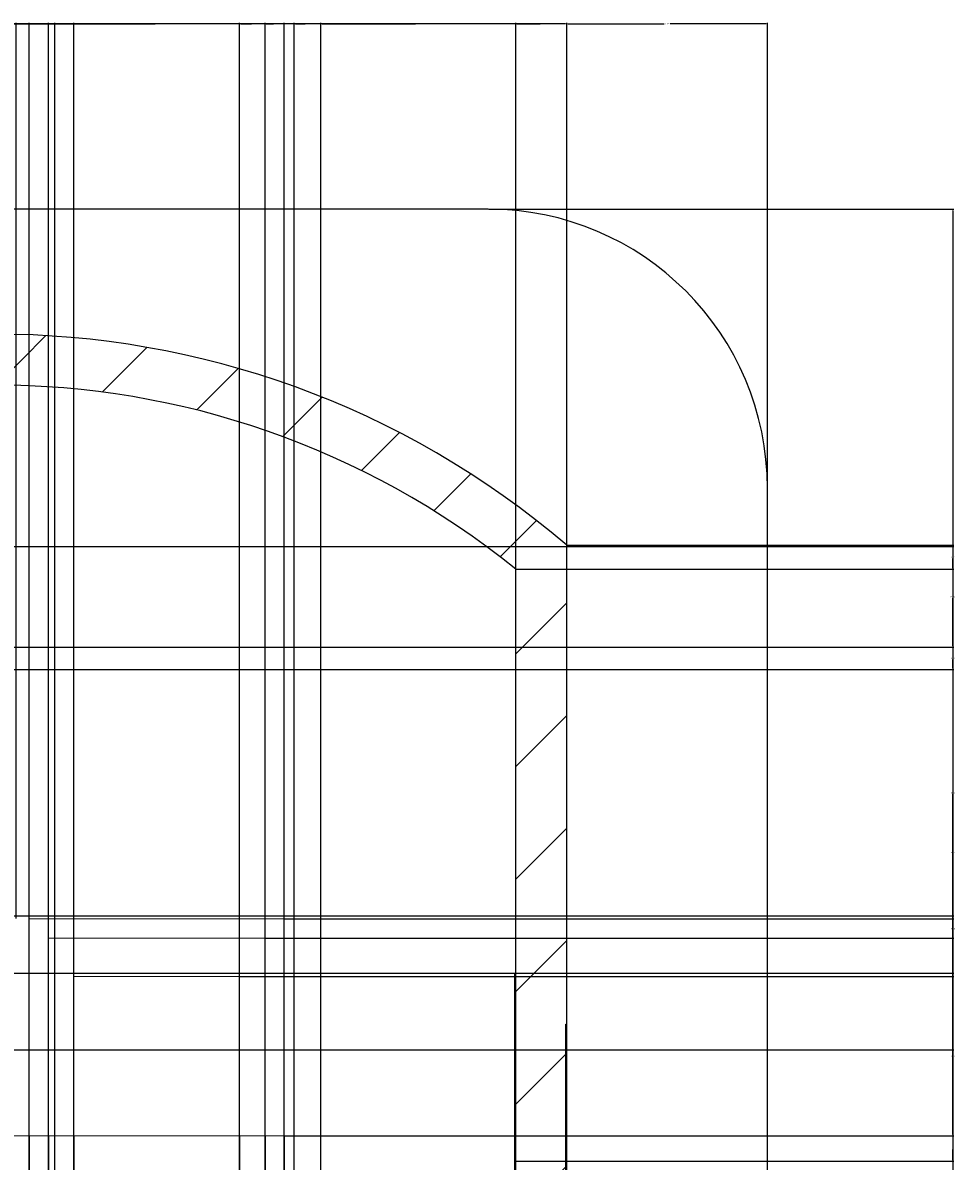
# Model space of a CAD drawing. Units: inches. Extents: x -14 to 375, y -86 to 549.
# Tile 12 of 12: x 228 to 375, y 336 to 515. Entities that reach past the tile are written whole.
import ezdxf

# ---------------------------------------------------------------- set-up
doc = ezdxf.new("R2010")
doc.units = ezdxf.units.IN
doc.header["$MEASUREMENT"] = 0
for name, color, linetype, lineweight in [('A-ANNO-DIMS', 2, 'Continuous', 18), ('A-DOOR', 3, 'Continuous', 18), ('A-ELEV', 7, 'Continuous', 25), ('A-ELEV-PATT', 8, 'Continuous', 13), ('A-ELEV-RAIL', 8, 'Continuous', 18)]:
    doc.layers.add(name, color=color, linetype=linetype, lineweight=lineweight)
doc.styles.get("Standard").update_dxf_attribs({"font": 'arial.ttf'})
doc.dimstyles.get("Standard").update_dxf_attribs({"dimtxt": 0.18, "dimasz": 0.18, "dimexe": 0.18, "dimexo": 0.0625, "dimgap": 0.09, "dimtad": 0, "dimtih": 1, "dimtoh": 1, "dimdec": 4, "dimzin": 0, "dimdsep": 46, "dimtxsty": 'Standard', "dimcen": 0.09, "dimadec": 0, "dimazin": 0, "dimtfac": 1, "dimtdec": 4, "dimtofl": 0, "dimtmove": 0, "dimatfit": 3, "dimfxl": 1, "dimtolj": 1, "dimtzin": 0, "dimarcsym": 0})

# ---------------------------------------------------------------- blocks, each defined once
blk = doc.blocks.new('*D8')
at = {"layer": 'A-ANNO-DIMS', "color": 0, "lineweight": -2, "transparency": 16777216}
for p, q in [((134.23, 433.23), (134.23, 515.24)), ((134.41, 515.06), (223.55, 515.06)), ((313.59, 515.06), (224.46, 515.06)), ((313.77, 433.23), (313.77, 515.24))]:
    blk.add_line(p, q, dxfattribs=at)
at = {"layer": 'A-ANNO-DIMS', "color": 0, "transparency": 16777216}
for points in [[(134.41, 515.09), (134.41, 515.03), (134.23, 515.06)], [(313.59, 515.09), (313.59, 515.03), (313.77, 515.06)]]:
    blk.add_solid(points, dxfattribs=at)
at = {"layer": 'Defpoints', "color": 0, "transparency": 16777216}
for p in [(313.77, 515.06), (134.23, 433.17), (313.77, 433.17)]:
    blk.add_point(p, dxfattribs=at)
at = {"layer": 'A-ANNO-DIMS', "color": 0, "transparency": 16777216, "insert": (224, 515.06), "char_height": 0.18, "attachment_point": 5}
blk.add_mtext('\\A1;179.54', dxfattribs=at)
blk = doc.blocks.new('*D9')
at = {"layer": 'A-ANNO-DIMS', "color": 0, "lineweight": -2, "transparency": 16777216}
for p, q in [((313.77, 433.23), (313.77, 515.24)), ((313.95, 515.06), (329.05, 515.06)), ((345.08, 515.06), (329.98, 515.06)), ((345.26, 442.21), (345.26, 515.24))]:
    blk.add_line(p, q, dxfattribs=at)
at = {"layer": 'A-ANNO-DIMS', "color": 0, "transparency": 16777216}
for points in [[(313.95, 515.09), (313.95, 515.03), (313.77, 515.06)], [(345.08, 515.09), (345.08, 515.03), (345.26, 515.06)]]:
    blk.add_solid(points, dxfattribs=at)
at = {"layer": 'Defpoints', "color": 0, "transparency": 16777216}
for p in [(345.26, 515.06), (345.26, 442.15), (313.77, 433.17)]:
    blk.add_point(p, dxfattribs=at)
at = {"layer": 'A-ANNO-DIMS', "color": 0, "transparency": 16777216, "insert": (329.52, 515.06), "char_height": 0.18, "attachment_point": 5}
blk.add_mtext('\\A1;31.495', dxfattribs=at)
blk = doc.blocks.new('*D10')
at = {"layer": 'A-ANNO-DIMS', "color": 0, "lineweight": -2, "transparency": 16777216}
for p, q in [((301.52, 485.96), (374.54, 485.96)), ((374.36, 485.78), (374.36, 225.61)), ((374.36, -34.93), (374.36, 225.24)), ((345.33, -35.11), (374.54, -35.11))]:
    blk.add_line(p, q, dxfattribs=at)
at = {"layer": 'A-ANNO-DIMS', "color": 0, "transparency": 16777216}
for points in [[(374.33, 485.78), (374.39, 485.78), (374.36, 485.96)], [(374.33, -34.93), (374.39, -34.93), (374.36, -35.11)]]:
    blk.add_solid(points, dxfattribs=at)
at = {"layer": 'Defpoints', "color": 0, "transparency": 16777216}
for p in [(301.46, 485.96), (374.36, 485.96), (345.26, -35.11)]:
    blk.add_point(p, dxfattribs=at)
at = {"layer": 'A-ANNO-DIMS', "color": 0, "transparency": 16777216, "insert": (374.36, 225.42), "char_height": 0.18, "attachment_point": 5}
blk.add_mtext('\\A1;521.1', dxfattribs=at)
blk = doc.blocks.new('*D36')
at = {"layer": 'A-ANNO-DIMS', "color": 0, "lineweight": -2, "transparency": 16777216}
for p, q in [((107.56, 353.96), (374.54, 353.96)), ((374.36, 353.78), (374.36, 327.93)), ((374.36, 301.72), (374.36, 327.57)), ((107.64, 301.54), (374.54, 301.54))]:
    blk.add_line(p, q, dxfattribs=at)
at = {"layer": 'A-ANNO-DIMS', "color": 0, "transparency": 16777216}
for points in [[(374.33, 353.78), (374.39, 353.78), (374.36, 353.96)], [(374.33, 301.72), (374.39, 301.72), (374.36, 301.54)]]:
    blk.add_solid(points, dxfattribs=at)
at = {"layer": 'Defpoints', "color": 0, "transparency": 16777216}
for p in [(107.5, 353.96), (374.36, 353.96), (107.58, 301.54)]:
    blk.add_point(p, dxfattribs=at)
at = {"layer": 'A-ANNO-DIMS', "color": 0, "transparency": 16777216, "insert": (374.36, 327.75), "char_height": 0.18, "attachment_point": 5}
blk.add_mtext('\\A1;52.42', dxfattribs=at)
blk = doc.blocks.new('*D37')
at = {"layer": 'A-ANNO-DIMS', "color": 0, "lineweight": -2, "transparency": 16777216}
for p, q in [((107.76, 365.96), (374.54, 365.96)), ((374.36, 365.78), (374.36, 360.14)), ((374.36, 354.14), (374.36, 359.78)), ((107.56, 353.96), (374.54, 353.96))]:
    blk.add_line(p, q, dxfattribs=at)
at = {"layer": 'A-ANNO-DIMS', "color": 0, "transparency": 16777216}
for points in [[(374.33, 365.78), (374.39, 365.78), (374.36, 365.96)], [(374.33, 354.14), (374.39, 354.14), (374.36, 353.96)]]:
    blk.add_solid(points, dxfattribs=at)
at = {"layer": 'Defpoints', "color": 0, "transparency": 16777216}
for p in [(107.7, 365.96), (374.36, 365.96), (107.5, 353.96)]:
    blk.add_point(p, dxfattribs=at)
at = {"layer": 'A-ANNO-DIMS', "color": 0, "transparency": 16777216, "insert": (374.36, 359.96), "char_height": 0.18, "attachment_point": 5}
blk.add_mtext('\\A1;12', dxfattribs=at)
blk = doc.blocks.new('*D38')
at = {"layer": 'A-ANNO-DIMS', "color": 0, "lineweight": -2, "transparency": 16777216}
for p, q in [((107.56, 374.96), (374.54, 374.96)), ((374.36, 374.78), (374.36, 370.64)), ((374.36, 366.14), (374.36, 370.28)), ((107.76, 365.96), (374.54, 365.96))]:
    blk.add_line(p, q, dxfattribs=at)
at = {"layer": 'A-ANNO-DIMS', "color": 0, "transparency": 16777216}
for points in [[(374.33, 374.78), (374.39, 374.78), (374.36, 374.96)], [(374.33, 366.14), (374.39, 366.14), (374.36, 365.96)]]:
    blk.add_solid(points, dxfattribs=at)
at = {"layer": 'Defpoints', "color": 0, "transparency": 16777216}
for p in [(107.5, 374.96), (374.36, 374.96), (107.7, 365.96)]:
    blk.add_point(p, dxfattribs=at)
at = {"layer": 'A-ANNO-DIMS', "color": 0, "transparency": 16777216, "insert": (374.36, 370.46), "char_height": 0.18, "attachment_point": 5}
blk.add_mtext('\\A1;9', dxfattribs=at)
blk = doc.blocks.new('*D39')
at = {"layer": 'A-ANNO-DIMS', "color": 0, "lineweight": -2, "transparency": 16777216}
for p, q in [((107.56, 413.68), (374.54, 413.68)), ((374.36, 413.5), (374.36, 394.5)), ((374.36, 375.14), (374.36, 394.14)), ((107.56, 374.96), (374.54, 374.96))]:
    blk.add_line(p, q, dxfattribs=at)
at = {"layer": 'A-ANNO-DIMS', "color": 0, "transparency": 16777216}
for points in [[(374.33, 413.5), (374.39, 413.5), (374.36, 413.68)], [(374.33, 375.14), (374.39, 375.14), (374.36, 374.96)]]:
    blk.add_solid(points, dxfattribs=at)
at = {"layer": 'Defpoints', "color": 0, "transparency": 16777216}
for p in [(107.5, 413.68), (374.36, 413.68), (107.5, 374.96)]:
    blk.add_point(p, dxfattribs=at)
at = {"layer": 'A-ANNO-DIMS', "color": 0, "transparency": 16777216, "insert": (374.36, 394.32), "char_height": 0.18, "attachment_point": 5}
blk.add_mtext('\\A1;38.72', dxfattribs=at)
blk = doc.blocks.new('*D40')
at = {"layer": 'A-ANNO-DIMS', "color": 0, "lineweight": -2, "transparency": 16777216}
for p, q in [((107.56, 417.18), (374.54, 417.18)), ((374.36, 417), (374.36, 415.61)), ((374.36, 413.86), (374.36, 415.25)), ((107.56, 413.68), (374.54, 413.68))]:
    blk.add_line(p, q, dxfattribs=at)
at = {"layer": 'A-ANNO-DIMS', "color": 0, "transparency": 16777216}
for points in [[(374.33, 417), (374.39, 417), (374.36, 417.18)], [(374.33, 413.86), (374.39, 413.86), (374.36, 413.68)]]:
    blk.add_solid(points, dxfattribs=at)
at = {"layer": 'Defpoints', "color": 0, "transparency": 16777216}
for p in [(107.5, 417.18), (374.36, 417.18), (107.5, 413.68)]:
    blk.add_point(p, dxfattribs=at)
at = {"layer": 'A-ANNO-DIMS', "color": 0, "transparency": 16777216, "insert": (374.36, 415.43), "char_height": 0.18, "attachment_point": 5}
blk.add_mtext('\\A1;3.501', dxfattribs=at)
blk = doc.blocks.new('*D41')
at = {"layer": 'A-ANNO-DIMS', "color": 0, "lineweight": -2, "transparency": 16777216}
for p, q in [((111.56, 432.97), (374.54, 432.97)), ((374.36, 432.79), (374.36, 425.26)), ((374.36, 417.36), (374.36, 424.89)), ((107.56, 417.18), (374.54, 417.18))]:
    blk.add_line(p, q, dxfattribs=at)
at = {"layer": 'A-ANNO-DIMS', "color": 0, "transparency": 16777216}
for points in [[(374.33, 432.79), (374.39, 432.79), (374.36, 432.97)], [(374.33, 417.36), (374.39, 417.36), (374.36, 417.18)]]:
    blk.add_solid(points, dxfattribs=at)
at = {"layer": 'Defpoints', "color": 0, "transparency": 16777216}
for p in [(111.5, 432.97), (374.36, 432.97), (107.5, 417.18)]:
    blk.add_point(p, dxfattribs=at)
at = {"layer": 'A-ANNO-DIMS', "color": 0, "transparency": 16777216, "insert": (374.36, 425.07), "char_height": 0.18, "attachment_point": 5}
blk.add_mtext('\\A1;15.786', dxfattribs=at)
blk = doc.blocks.new('*D55')
at = {"layer": 'A-ANNO-DIMS', "color": 0, "lineweight": -2, "transparency": 16777216}
for p, q in [((227.37, 374.55), (227.37, 515.24)), ((227.55, 515.06), (228.06, 515.06)), ((229.23, 515.06), (228.71, 515.06)), ((229.41, 374.55), (229.41, 515.24))]:
    blk.add_line(p, q, dxfattribs=at)
at = {"layer": 'A-ANNO-DIMS', "color": 0, "transparency": 16777216}
for points in [[(227.55, 515.09), (227.55, 515.03), (227.37, 515.06)], [(229.23, 515.09), (229.23, 515.03), (229.41, 515.06)]]:
    blk.add_solid(points, dxfattribs=at)
at = {"layer": 'Defpoints', "color": 0, "transparency": 16777216}
for p in [(229.41, 515.06), (227.37, 374.49), (229.41, 374.49)]:
    blk.add_point(p, dxfattribs=at)
at = {"layer": 'A-ANNO-DIMS', "color": 0, "transparency": 16777216, "insert": (228.39, 515.06), "char_height": 0.18, "attachment_point": 5}
blk.add_mtext('\\A1;2.04', dxfattribs=at)
blk = doc.blocks.new('*D56')
at = {"layer": 'A-ANNO-DIMS', "color": 0, "lineweight": -2, "transparency": 16777216}
for p, q in [((229.41, 374.55), (229.41, 515.24)), ((229.59, 515.06), (249.19, 515.06)), ((269.23, 515.06), (249.63, 515.06)), ((269.41, 374.55), (269.41, 515.24))]:
    blk.add_line(p, q, dxfattribs=at)
at = {"layer": 'A-ANNO-DIMS', "color": 0, "transparency": 16777216}
for points in [[(229.59, 515.09), (229.59, 515.03), (229.41, 515.06)], [(269.23, 515.09), (269.23, 515.03), (269.41, 515.06)]]:
    blk.add_solid(points, dxfattribs=at)
at = {"layer": 'Defpoints', "color": 0, "transparency": 16777216}
for p in [(269.41, 515.06), (229.41, 374.49), (269.41, 374.49)]:
    blk.add_point(p, dxfattribs=at)
at = {"layer": 'A-ANNO-DIMS', "color": 0, "transparency": 16777216, "insert": (249.41, 515.06), "char_height": 0.18, "attachment_point": 5}
blk.add_mtext('\\A1;40', dxfattribs=at)
blk = doc.blocks.new('*D57')
at = {"layer": 'A-ANNO-DIMS', "color": 0, "lineweight": -2, "transparency": 16777216}
for p, q in [((229.41, 340.38), (229.41, -64.39)), ((232.41, 340.38), (232.41, -64.39)), ((229.59, -64.21), (230.76, -64.21)), ((232.23, -64.21), (231.06, -64.21))]:
    blk.add_line(p, q, dxfattribs=at)
at = {"layer": 'A-ANNO-DIMS', "color": 0, "transparency": 16777216}
for points in [[(229.59, -64.18), (229.59, -64.24), (229.41, -64.21)], [(232.23, -64.18), (232.23, -64.24), (232.41, -64.21)]]:
    blk.add_solid(points, dxfattribs=at)
at = {"layer": 'Defpoints', "color": 0, "transparency": 16777216}
for p in [(229.41, 340.44), (232.41, 340.44), (232.41, -64.21)]:
    blk.add_point(p, dxfattribs=at)
at = {"layer": 'A-ANNO-DIMS', "color": 0, "transparency": 16777216, "insert": (230.91, -64.21), "char_height": 0.18, "attachment_point": 5}
blk.add_mtext('\\A1;3', dxfattribs=at)
blk = doc.blocks.new('*D58')
at = {"layer": 'A-ANNO-DIMS', "color": 0, "lineweight": -2, "transparency": 16777216}
for p, q in [((232.41, 340.38), (232.41, -64.39)), ((236.41, 340.38), (236.41, -64.39)), ((232.59, -64.21), (234.26, -64.21)), ((236.23, -64.21), (234.56, -64.21))]:
    blk.add_line(p, q, dxfattribs=at)
at = {"layer": 'A-ANNO-DIMS', "color": 0, "transparency": 16777216}
for points in [[(232.59, -64.18), (232.59, -64.24), (232.41, -64.21)], [(236.23, -64.18), (236.23, -64.24), (236.41, -64.21)]]:
    blk.add_solid(points, dxfattribs=at)
at = {"layer": 'Defpoints', "color": 0, "transparency": 16777216}
for p in [(232.41, 340.44), (236.41, 340.44), (236.41, -64.21)]:
    blk.add_point(p, dxfattribs=at)
at = {"layer": 'A-ANNO-DIMS', "color": 0, "transparency": 16777216, "insert": (234.41, -64.21), "char_height": 0.18, "attachment_point": 5}
blk.add_mtext('\\A1;4', dxfattribs=at)
blk = doc.blocks.new('*D59')
at = {"layer": 'A-ANNO-DIMS', "color": 0, "lineweight": -2, "transparency": 16777216}
for p, q in [((236.41, 340.38), (236.41, -64.39)), ((262.41, 340.38), (262.41, -64.39)), ((236.59, -64.21), (249.19, -64.21)), ((262.23, -64.21), (249.63, -64.21))]:
    blk.add_line(p, q, dxfattribs=at)
at = {"layer": 'A-ANNO-DIMS', "color": 0, "transparency": 16777216}
for points in [[(236.59, -64.18), (236.59, -64.24), (236.41, -64.21)], [(262.23, -64.18), (262.23, -64.24), (262.41, -64.21)]]:
    blk.add_solid(points, dxfattribs=at)
at = {"layer": 'Defpoints', "color": 0, "transparency": 16777216}
for p in [(236.41, 340.44), (262.41, 340.44), (262.41, -64.21)]:
    blk.add_point(p, dxfattribs=at)
at = {"layer": 'A-ANNO-DIMS', "color": 0, "transparency": 16777216, "insert": (249.41, -64.21), "char_height": 0.18, "attachment_point": 5}
blk.add_mtext('\\A1;26', dxfattribs=at)
blk = doc.blocks.new('*D60')
at = {"layer": 'A-ANNO-DIMS', "color": 0, "lineweight": -2, "transparency": 16777216}
for p, q in [((262.41, 340.38), (262.41, -64.39)), ((266.41, 340.38), (266.41, -64.39)), ((262.59, -64.21), (264.26, -64.21)), ((266.23, -64.21), (264.56, -64.21))]:
    blk.add_line(p, q, dxfattribs=at)
at = {"layer": 'A-ANNO-DIMS', "color": 0, "transparency": 16777216}
for points in [[(262.59, -64.18), (262.59, -64.24), (262.41, -64.21)], [(266.23, -64.18), (266.23, -64.24), (266.41, -64.21)]]:
    blk.add_solid(points, dxfattribs=at)
at = {"layer": 'Defpoints', "color": 0, "transparency": 16777216}
for p in [(262.41, 340.44), (266.41, 340.44), (266.41, -64.21)]:
    blk.add_point(p, dxfattribs=at)
at = {"layer": 'A-ANNO-DIMS', "color": 0, "transparency": 16777216, "insert": (264.41, -64.21), "char_height": 0.18, "attachment_point": 5}
blk.add_mtext('\\A1;4', dxfattribs=at)
blk = doc.blocks.new('*D61')
at = {"layer": 'A-ANNO-DIMS', "color": 0, "lineweight": -2, "transparency": 16777216}
for p, q in [((266.41, 340.38), (266.41, -64.39)), ((269.41, 340.38), (269.41, -64.39)), ((266.59, -64.21), (267.76, -64.21)), ((269.23, -64.21), (268.06, -64.21))]:
    blk.add_line(p, q, dxfattribs=at)
at = {"layer": 'A-ANNO-DIMS', "color": 0, "transparency": 16777216}
for points in [[(266.59, -64.18), (266.59, -64.24), (266.41, -64.21)], [(269.23, -64.18), (269.23, -64.24), (269.41, -64.21)]]:
    blk.add_solid(points, dxfattribs=at)
at = {"layer": 'Defpoints', "color": 0, "transparency": 16777216}
for p in [(266.41, 340.44), (269.41, 340.44), (269.41, -64.21)]:
    blk.add_point(p, dxfattribs=at)
at = {"layer": 'A-ANNO-DIMS', "color": 0, "transparency": 16777216, "insert": (267.91, -64.21), "char_height": 0.18, "attachment_point": 5}
blk.add_mtext('\\A1;3', dxfattribs=at)
blk = doc.blocks.new('*D64')
at = {"layer": 'A-ANNO-DIMS', "color": 0, "lineweight": -2, "transparency": 16777216}
for p, q in [((305.69, 336.44), (374.54, 336.44)), ((374.36, 336.26), (374.36, 321.76)), ((374.36, 306.89), (374.36, 321.39)), ((305.69, 306.71), (374.54, 306.71))]:
    blk.add_line(p, q, dxfattribs=at)
at = {"layer": 'A-ANNO-DIMS', "color": 0, "transparency": 16777216}
for points in [[(374.33, 336.26), (374.39, 336.26), (374.36, 336.44)], [(374.33, 306.89), (374.39, 306.89), (374.36, 306.71)]]:
    blk.add_solid(points, dxfattribs=at)
at = {"layer": 'Defpoints', "color": 0, "transparency": 16777216}
for p in [(305.63, 336.44), (374.36, 336.44), (305.63, 306.71)]:
    blk.add_point(p, dxfattribs=at)
at = {"layer": 'A-ANNO-DIMS', "color": 0, "transparency": 16777216, "insert": (374.36, 321.57), "char_height": 0.18, "attachment_point": 5}
blk.add_mtext('\\A1;29.735', dxfattribs=at)
blk = doc.blocks.new('*D65')
at = {"layer": 'A-ANNO-DIMS', "color": 0, "lineweight": -2, "transparency": 16777216}
for p, q in [((305.690578, 340.442088), (374.544714, 340.442088)), ((374.364714, 340.262088), (374.364714, 338.622088)), ((374.364714, 336.622088), (374.364714, 338.262088)), ((305.690578, 336.442088), (374.544714, 336.442088))]:
    blk.add_line(p, q, dxfattribs=at)
at = {"layer": 'A-ANNO-DIMS', "color": 0, "transparency": 16777216}
for points in [[(374.334714, 340.262088), (374.394714, 340.262088), (374.364714, 340.442088)], [(374.334714, 336.622088), (374.394714, 336.622088), (374.364714, 336.442088)]]:
    blk.add_solid(points, dxfattribs=at)
at = {"layer": 'Defpoints', "color": 0, "transparency": 16777216}
for p in [(305.628078, 340.442088), (374.364714, 340.442088), (305.628078, 336.442088)]:
    blk.add_point(p, dxfattribs=at)
at = {"layer": 'A-ANNO-DIMS', "color": 0, "transparency": 16777216, "insert": (374.364714, 338.442088), "char_height": 0.18, "attachment_point": 5}
blk.add_mtext('\\A1;4', dxfattribs=at)
blk = doc.blocks.new('*D66')
at = {"layer": 'A-ANNO-DIMS', "color": 0, "lineweight": -2, "transparency": 16777216}
for p, q in [((305.83, 429.42), (374.54, 429.42)), ((374.36, 429.24), (374.36, 385.11)), ((374.36, 340.62), (374.36, 384.75)), ((305.69, 340.44), (374.54, 340.44))]:
    blk.add_line(p, q, dxfattribs=at)
at = {"layer": 'A-ANNO-DIMS', "color": 0, "transparency": 16777216}
for points in [[(374.33, 429.24), (374.39, 429.24), (374.36, 429.42)], [(374.33, 340.62), (374.39, 340.62), (374.36, 340.44)]]:
    blk.add_solid(points, dxfattribs=at)
at = {"layer": 'Defpoints', "color": 0, "transparency": 16777216}
for p in [(305.77, 429.42), (374.36, 429.42), (305.63, 340.44)]:
    blk.add_point(p, dxfattribs=at)
at = {"layer": 'A-ANNO-DIMS', "color": 0, "transparency": 16777216, "insert": (374.36, 384.93), "char_height": 0.18, "attachment_point": 5}
blk.add_mtext('\\A1;88.98', dxfattribs=at)
blk = doc.blocks.new('*D67')
at = {"layer": 'A-ANNO-DIMS', "color": 0, "lineweight": -2, "transparency": 16777216}
for p, q in [((313.83, 433.17), (374.54, 433.17)), ((374.36, 432.99), (374.36, 431.48)), ((374.36, 429.6), (374.36, 431.11)), ((305.83, 429.42), (374.54, 429.42))]:
    blk.add_line(p, q, dxfattribs=at)
at = {"layer": 'A-ANNO-DIMS', "color": 0, "transparency": 16777216}
for points in [[(374.33, 432.99), (374.39, 432.99), (374.36, 433.17)], [(374.33, 429.6), (374.39, 429.6), (374.36, 429.42)]]:
    blk.add_solid(points, dxfattribs=at)
at = {"layer": 'Defpoints', "color": 0, "transparency": 16777216}
for p in [(313.77, 433.17), (374.36, 433.17), (305.77, 429.42)]:
    blk.add_point(p, dxfattribs=at)
at = {"layer": 'A-ANNO-DIMS', "color": 0, "transparency": 16777216, "insert": (374.36, 431.3), "char_height": 0.18, "attachment_point": 5}
blk.add_mtext('\\A1;3.751', dxfattribs=at)
blk = doc.blocks.new('*D68')
at = {"layer": 'A-ANNO-DIMS', "color": 0, "lineweight": -2, "transparency": 16777216}
for p, q in [((262.47, 365.46), (374.54, 365.46)), ((374.36, 365.28), (374.36, 353.13)), ((374.36, 340.62), (374.36, 352.77)), ((269.47, 340.44), (374.54, 340.44))]:
    blk.add_line(p, q, dxfattribs=at)
at = {"layer": 'A-ANNO-DIMS', "color": 0, "transparency": 16777216}
for points in [[(374.33, 365.28), (374.39, 365.28), (374.36, 365.46)], [(374.33, 340.62), (374.39, 340.62), (374.36, 340.44)]]:
    blk.add_solid(points, dxfattribs=at)
at = {"layer": 'Defpoints', "color": 0, "transparency": 16777216}
for p in [(262.41, 365.46), (374.36, 365.46), (269.41, 340.44)]:
    blk.add_point(p, dxfattribs=at)
at = {"layer": 'A-ANNO-DIMS', "color": 0, "transparency": 16777216, "insert": (374.36, 352.95), "char_height": 0.18, "attachment_point": 5}
blk.add_mtext('\\A1;25.02', dxfattribs=at)
blk = doc.blocks.new('*D69')
at = {"layer": 'A-ANNO-DIMS', "color": 0, "lineweight": -2, "transparency": 16777216}
for p, q in [((266.47, 371.46), (374.54, 371.46)), ((374.36, 371.28), (374.36, 368.64)), ((374.36, 365.64), (374.36, 368.28)), ((262.47, 365.46), (374.54, 365.46))]:
    blk.add_line(p, q, dxfattribs=at)
at = {"layer": 'A-ANNO-DIMS', "color": 0, "transparency": 16777216}
for points in [[(374.33, 371.28), (374.39, 371.28), (374.36, 371.46)], [(374.33, 365.64), (374.39, 365.64), (374.36, 365.46)]]:
    blk.add_solid(points, dxfattribs=at)
at = {"layer": 'Defpoints', "color": 0, "transparency": 16777216}
for p in [(266.41, 371.46), (374.36, 371.46), (262.41, 365.46)]:
    blk.add_point(p, dxfattribs=at)
at = {"layer": 'A-ANNO-DIMS', "color": 0, "transparency": 16777216, "insert": (374.36, 368.46), "char_height": 0.18, "attachment_point": 5}
blk.add_mtext('\\A1;6', dxfattribs=at)
blk = doc.blocks.new('*D70')
at = {"layer": 'A-ANNO-DIMS', "color": 0, "lineweight": -2, "transparency": 16777216}
for p, q in [((269.47, 374.49), (374.54, 374.49)), ((374.36, 374.31), (374.36, 373.16)), ((374.36, 371.64), (374.36, 372.79)), ((266.47, 371.46), (374.54, 371.46))]:
    blk.add_line(p, q, dxfattribs=at)
at = {"layer": 'A-ANNO-DIMS', "color": 0, "transparency": 16777216}
for points in [[(374.33, 374.31), (374.39, 374.31), (374.36, 374.49)], [(374.33, 371.64), (374.39, 371.64), (374.36, 371.46)]]:
    blk.add_solid(points, dxfattribs=at)
at = {"layer": 'Defpoints', "color": 0, "transparency": 16777216}
for p in [(269.41, 374.49), (374.36, 374.49), (266.41, 371.46)]:
    blk.add_point(p, dxfattribs=at)
at = {"layer": 'A-ANNO-DIMS', "color": 0, "transparency": 16777216, "insert": (374.36, 372.97), "char_height": 0.18, "attachment_point": 5}
blk.add_mtext('\\A1;3.023', dxfattribs=at)
blk = doc.blocks.new('*D72')
at = {"layer": 'A-ANNO-DIMS', "color": 0, "lineweight": -2, "transparency": 16777216}
for p, q in [((229.41, 126.03), (229.41, 515.24)), ((229.59, 515.06), (231.26, 515.06)), ((233.23, 515.06), (231.56, 515.06)), ((233.41, 168.03), (233.41, 515.24))]:
    blk.add_line(p, q, dxfattribs=at)
at = {"layer": 'A-ANNO-DIMS', "color": 0, "transparency": 16777216}
for points in [[(229.59, 515.09), (229.59, 515.03), (229.41, 515.06)], [(233.23, 515.09), (233.23, 515.03), (233.41, 515.06)]]:
    blk.add_solid(points, dxfattribs=at)
at = {"layer": 'Defpoints', "color": 0, "transparency": 16777216}
for p in [(233.41, 515.06), (233.41, 167.97), (229.41, 125.97)]:
    blk.add_point(p, dxfattribs=at)
at = {"layer": 'A-ANNO-DIMS', "color": 0, "transparency": 16777216, "insert": (231.41, 515.06), "char_height": 0.18, "attachment_point": 5}
blk.add_mtext('\\A1;4', dxfattribs=at)
blk = doc.blocks.new('*D85')
at = {"layer": 'A-ANNO-DIMS', "color": 0, "lineweight": -2, "transparency": 16777216}
for p, q in [((229.41, 210.03), (229.41, 515.24)), ((229.59, 515.06), (230.76, 515.06)), ((232.23, 515.06), (231.06, 515.06)), ((232.41, 207.01), (232.41, 515.24))]:
    blk.add_line(p, q, dxfattribs=at)
at = {"layer": 'A-ANNO-DIMS', "color": 0, "transparency": 16777216}
for points in [[(229.59, 515.09), (229.59, 515.03), (229.41, 515.06)], [(232.23, 515.09), (232.23, 515.03), (232.41, 515.06)]]:
    blk.add_solid(points, dxfattribs=at)
at = {"layer": 'Defpoints', "color": 0, "transparency": 16777216}
for p in [(232.41, 515.06), (229.41, 209.97), (232.41, 206.95)]:
    blk.add_point(p, dxfattribs=at)
at = {"layer": 'A-ANNO-DIMS', "color": 0, "transparency": 16777216, "insert": (230.91, 515.06), "char_height": 0.18, "attachment_point": 5}
blk.add_mtext('\\A1;3', dxfattribs=at)
blk = doc.blocks.new('*D86')
at = {"layer": 'A-ANNO-DIMS', "color": 0, "lineweight": -2, "transparency": 16777216}
for p, q in [((232.41, 207.01), (232.41, 515.24)), ((232.59, 515.06), (234.26, 515.06)), ((236.23, 515.06), (234.56, 515.06)), ((236.41, 201.01), (236.41, 515.24))]:
    blk.add_line(p, q, dxfattribs=at)
at = {"layer": 'A-ANNO-DIMS', "color": 0, "transparency": 16777216}
for points in [[(232.59, 515.09), (232.59, 515.03), (232.41, 515.06)], [(236.23, 515.09), (236.23, 515.03), (236.41, 515.06)]]:
    blk.add_solid(points, dxfattribs=at)
at = {"layer": 'Defpoints', "color": 0, "transparency": 16777216}
for p in [(236.41, 515.06), (232.41, 206.95), (236.41, 200.95)]:
    blk.add_point(p, dxfattribs=at)
at = {"layer": 'A-ANNO-DIMS', "color": 0, "transparency": 16777216, "insert": (234.41, 515.06), "char_height": 0.18, "attachment_point": 5}
blk.add_mtext('\\A1;4', dxfattribs=at)
blk = doc.blocks.new('*D87')
at = {"layer": 'A-ANNO-DIMS', "color": 0, "lineweight": -2, "transparency": 16777216}
for p, q in [((236.41, 201.01), (236.41, 515.24)), ((236.59, 515.06), (249.19, 515.06)), ((262.23, 515.06), (249.63, 515.06)), ((262.41, 201.01), (262.41, 515.24))]:
    blk.add_line(p, q, dxfattribs=at)
at = {"layer": 'A-ANNO-DIMS', "color": 0, "transparency": 16777216}
for points in [[(236.59, 515.09), (236.59, 515.03), (236.41, 515.06)], [(262.23, 515.09), (262.23, 515.03), (262.41, 515.06)]]:
    blk.add_solid(points, dxfattribs=at)
at = {"layer": 'Defpoints', "color": 0, "transparency": 16777216}
for p in [(262.41, 515.06), (236.41, 200.95), (262.41, 200.95)]:
    blk.add_point(p, dxfattribs=at)
at = {"layer": 'A-ANNO-DIMS', "color": 0, "transparency": 16777216, "insert": (249.41, 515.06), "char_height": 0.18, "attachment_point": 5}
blk.add_mtext('\\A1;26', dxfattribs=at)
blk = doc.blocks.new('*D88')
at = {"layer": 'A-ANNO-DIMS', "color": 0, "lineweight": -2, "transparency": 16777216}
for p, q in [((262.41, 201.01), (262.41, 515.24)), ((262.59, 515.06), (264.26, 515.06)), ((266.23, 515.06), (264.56, 515.06)), ((266.41, 207.01), (266.41, 515.24))]:
    blk.add_line(p, q, dxfattribs=at)
at = {"layer": 'A-ANNO-DIMS', "color": 0, "transparency": 16777216}
for points in [[(262.59, 515.09), (262.59, 515.03), (262.41, 515.06)], [(266.23, 515.09), (266.23, 515.03), (266.41, 515.06)]]:
    blk.add_solid(points, dxfattribs=at)
at = {"layer": 'Defpoints', "color": 0, "transparency": 16777216}
for p in [(266.41, 515.06), (266.41, 206.95), (262.41, 200.95)]:
    blk.add_point(p, dxfattribs=at)
at = {"layer": 'A-ANNO-DIMS', "color": 0, "transparency": 16777216, "insert": (264.41, 515.06), "char_height": 0.18, "attachment_point": 5}
blk.add_mtext('\\A1;4', dxfattribs=at)
blk = doc.blocks.new('*D89')
at = {"layer": 'A-ANNO-DIMS', "color": 0, "lineweight": -2, "transparency": 16777216}
for p, q in [((266.41, 207.01), (266.41, 515.24)), ((266.59, 515.06), (267.76, 515.06)), ((269.23, 515.06), (268.06, 515.06)), ((269.41, 210.03), (269.41, 515.24))]:
    blk.add_line(p, q, dxfattribs=at)
at = {"layer": 'A-ANNO-DIMS', "color": 0, "transparency": 16777216}
for points in [[(266.59, 515.09), (266.59, 515.03), (266.41, 515.06)], [(269.23, 515.09), (269.23, 515.03), (269.41, 515.06)]]:
    blk.add_solid(points, dxfattribs=at)
at = {"layer": 'Defpoints', "color": 0, "transparency": 16777216}
for p in [(269.41, 515.06), (269.41, 209.97), (266.41, 206.95)]:
    blk.add_point(p, dxfattribs=at)
at = {"layer": 'A-ANNO-DIMS', "color": 0, "transparency": 16777216, "insert": (267.91, 515.06), "char_height": 0.18, "attachment_point": 5}
blk.add_mtext('\\A1;3', dxfattribs=at)
blk = doc.blocks.new('*D104')
at = {"layer": 'A-ANNO-DIMS', "color": 0, "lineweight": -2, "transparency": 16777216}
for p, q in [((190.15, 6.02), (190.15, 515.24)), ((190.33, 515.06), (230.18, 515.06)), ((270.82, 515.06), (230.97, 515.06)), ((271, 6.02), (271, 515.24))]:
    blk.add_line(p, q, dxfattribs=at)
at = {"layer": 'A-ANNO-DIMS', "color": 0, "transparency": 16777216}
for points in [[(190.33, 515.09), (190.33, 515.03), (190.15, 515.06)], [(270.82, 515.09), (270.82, 515.03), (271, 515.06)]]:
    blk.add_solid(points, dxfattribs=at)
at = {"layer": 'Defpoints', "color": 0, "transparency": 16777216}
for p in [(271, 515.06), (190.15, 5.96), (271, 5.96)]:
    blk.add_point(p, dxfattribs=at)
at = {"layer": 'A-ANNO-DIMS', "color": 0, "transparency": 16777216, "insert": (230.57, 515.06), "char_height": 0.18, "attachment_point": 5}
blk.add_mtext('\\A1;80.85', dxfattribs=at)
blk = doc.blocks.new('*D105')
at = {"layer": 'A-ANNO-DIMS', "color": 0, "lineweight": -2, "transparency": 16777216}
for p, q in [((271, 6.02), (271, 515.24)), ((271.18, 515.06), (272.69, 515.06)), ((275.01, 515.06), (273.49, 515.06)), ((275.19, 6.02), (275.19, 515.24))]:
    blk.add_line(p, q, dxfattribs=at)
at = {"layer": 'A-ANNO-DIMS', "color": 0, "transparency": 16777216}
for points in [[(271.18, 515.09), (271.18, 515.03), (271, 515.06)], [(275.01, 515.09), (275.01, 515.03), (275.19, 515.06)]]:
    blk.add_solid(points, dxfattribs=at)
at = {"layer": 'Defpoints', "color": 0, "transparency": 16777216}
for p in [(275.19, 515.06), (271, 5.96), (275.19, 5.96)]:
    blk.add_point(p, dxfattribs=at)
at = {"layer": 'A-ANNO-DIMS', "color": 0, "transparency": 16777216, "insert": (273.09, 515.06), "char_height": 0.18, "attachment_point": 5}
blk.add_mtext('\\A1;4.186', dxfattribs=at)
blk = doc.blocks.new('*D106')
at = {"layer": 'A-ANNO-DIMS', "color": 0, "lineweight": -2, "transparency": 16777216}
for p, q in [((275.19, 6.02), (275.19, 515.24)), ((275.37, 515.06), (290.01, 515.06)), ((305.59, 515.06), (290.94, 515.06)), ((305.77, 6.02), (305.77, 515.24))]:
    blk.add_line(p, q, dxfattribs=at)
at = {"layer": 'A-ANNO-DIMS', "color": 0, "transparency": 16777216}
for points in [[(275.37, 515.09), (275.37, 515.03), (275.19, 515.06)], [(305.59, 515.09), (305.59, 515.03), (305.77, 515.06)]]:
    blk.add_solid(points, dxfattribs=at)
at = {"layer": 'Defpoints', "color": 0, "transparency": 16777216}
for p in [(305.77, 515.06), (275.19, 5.96), (305.77, 5.96)]:
    blk.add_point(p, dxfattribs=at)
at = {"layer": 'A-ANNO-DIMS', "color": 0, "transparency": 16777216, "insert": (290.48, 515.06), "char_height": 0.18, "attachment_point": 5}
blk.add_mtext('\\A1;30.585', dxfattribs=at)
blk = doc.blocks.new('*D107')
at = {"layer": 'A-ANNO-DIMS', "color": 0, "lineweight": -2, "transparency": 16777216}
for p, q in [((305.77, 6.02), (305.77, 515.24)), ((305.95, 515.06), (309.62, 515.06)), ((313.59, 515.06), (309.92, 515.06)), ((313.77, 6.02), (313.77, 515.24))]:
    blk.add_line(p, q, dxfattribs=at)
at = {"layer": 'A-ANNO-DIMS', "color": 0, "transparency": 16777216}
for points in [[(305.95, 515.09), (305.95, 515.03), (305.77, 515.06)], [(313.59, 515.09), (313.59, 515.03), (313.77, 515.06)]]:
    blk.add_solid(points, dxfattribs=at)
at = {"layer": 'Defpoints', "color": 0, "transparency": 16777216}
for p in [(313.77, 515.06), (305.77, 5.96), (313.77, 5.96)]:
    blk.add_point(p, dxfattribs=at)
at = {"layer": 'A-ANNO-DIMS', "color": 0, "transparency": 16777216, "insert": (309.77, 515.06), "char_height": 0.18, "attachment_point": 5}
blk.add_mtext('\\A1;8', dxfattribs=at)

msp = doc.modelspace()

# ---------------------------------------------------------------- hatches: boundary and pattern name
at = {"layer": 'A-ELEV-PATT'}
h = msp.add_hatch(dxfattribs=at)
h.set_pattern_fill('ANSI31', color=256, scale=100)
h.set_pattern_definition([(45, (-168.406, -22.703), (-8.83883, 8.83883), [])])
h.paths.add_polyline_path([(313.6281, 262.7071), (313.6281, 357.9589), (313.7701, 357.9589), (313.7701, 433.1717, 0.36940998), (134.2334, 433.1717), (134.2334, 365.9589), (134.2334, 262.7071)])
h.paths.add_polyline_path([(142.2334, 270.7071), (142.2334, 365.9589), (142.2334, 429.4208, -0.35358711), (305.7701, 429.4208), (305.7701, 365.9589), (305.6281, 365.9589), (305.6281, 270.7071)], flags=16)
h.paths.add_polyline_path([(134.2334, 187.8466), (134.2334, 117.9589), (313.7701, 117.9589), (313.7701, 187.8466, 0.62486768)])
h.paths.add_polyline_path([(305.7701, 185.9589), (305.7701, 125.9589), (142.2334, 125.9589), (142.2334, 185.9589, -0.61125102)], flags=16)
h.paths.add_polyline_path([(134.2334, 73.1717), (134.2334, 5.9589), (142.2334, 5.9589), (142.2334, 69.4208, -0.35358711), (305.7701, 69.4208), (305.7701, 5.9589), (313.7701, 5.9589), (313.7701, 73.1717, 0.36940998)])

# ---------------------------------------------------------------- linework, layer by layer
at = {"layer": 'A-DOOR'}
for p, q in [((305.7701, 365.9589), (305.6281, 365.9589)), ((305.6281, 365.9589), (305.7701, 365.9589))]:
    msp.add_line(p, q, dxfattribs=at)
for points in [[(269.409, 340.4421), (269.409, 374.4857), (229.409, 374.4857), (229.409, 340.4421)], [(266.409, 340.4421), (266.409, 371.4627), (232.409, 371.4627), (232.409, 340.4421)], [(236.409, 340.4421), (236.409, 365.4627), (262.409, 365.4627), (262.409, 340.4421)]]:
    msp.add_lwpolyline(points, dxfattribs=at)
at = {"layer": 'A-ELEV'}
msp.add_line((301.4553, 485.9589), (59.2112, 485.9589), dxfattribs=at)
msp.add_lwpolyline([(345.2647, 5.9589), (345.2647, 125.9589), (345.2647, 245.9589), (345.2647, 365.9589), (345.2647, 442.1495, 0.41421356), (301.4553, 485.9589)], format="xyb", dxfattribs=at)
for points in [[(134.2334, 262.7071), (313.6281, 262.7071), (313.6281, 357.9589), (313.7701, 357.9589), (313.7701, 433.1717, 0.36940998), (134.2334, 433.1717), (134.2334, 365.9589)], [(142.2334, 270.7071), (305.6281, 270.7071), (305.6281, 365.9589), (305.7701, 365.9589), (305.7701, 429.4208, 0.35358711), (142.2334, 429.4208), (142.2334, 365.9589)]]:
    msp.add_lwpolyline(points, format="xyb", close=True, dxfattribs=at)
at = {"layer": 'A-ELEV-RAIL'}
msp.add_line((305.6281, 340.4421), (142.2334, 340.4421), dxfattribs=at)

# ---------------------------------------------------------------- dimensions: what is measured, and where the dimension line sits
at = {"layer": 'A-ANNO-DIMS'}
for base, p1, p2, override, picture, middle in [((313.7701, 515.0589), (134.2334, 433.1717), (313.7701, 433.1717), {"dimdec": 2, "dimlfac": 1, "dimrnd": 0, "dimzin": 0, "dimdsep": 46, "dimlunit": 2}, '*D8', (224.0017, 515.0589)), ((270.9993, 515.0589), (190.148, 5.9589), (270.9993, 5.9589), {"dimdec": 2, "dimlfac": 1, "dimrnd": 0, "dimzin": 0, "dimdsep": 46, "dimlunit": 2}, '*D104', (230.5736, 515.0589)), ((229.409, 515.0589), (227.3657, 374.4857), (229.409, 374.4857), {"dimdec": 2, "dimlfac": 1, "dimrnd": 0, "dimzin": 0, "dimdsep": 46, "dimlunit": 2}, '*D55', (228.3874, 515.0589)), ((269.409, 515.0589), (229.409, 374.4857), (269.409, 374.4857), {"dimdec": 0, "dimlfac": 1, "dimrnd": 0, "dimzin": 0, "dimdsep": 46, "dimlunit": 2}, '*D56', (249.409, 515.0589)), ((233.409, 515.0589), (229.409, 125.9717), (233.409, 167.9717), {"dimdec": 0, "dimlfac": 1, "dimrnd": 0, "dimzin": 0, "dimdsep": 46, "dimlunit": 2}, '*D72', (231.409, 515.0589)), ((232.409, 515.0589), (229.409, 209.9717), (232.409, 206.9487), {"dimdec": 0, "dimlfac": 1, "dimrnd": 0, "dimzin": 0, "dimdsep": 46, "dimlunit": 2}, '*D85', (230.909, 515.0589)), ((236.409, 515.0589), (232.409, 206.9487), (236.409, 200.9487), {"dimdec": 0, "dimlfac": 1, "dimrnd": 0, "dimzin": 0, "dimdsep": 46, "dimlunit": 2}, '*D86', (234.409, 515.0589)), ((262.409, 515.0589), (236.409, 200.9487), (262.409, 200.9487), {"dimdec": 0, "dimlfac": 1, "dimrnd": 0, "dimzin": 0, "dimdsep": 46, "dimlunit": 2}, '*D87', (249.409, 515.0589)), ((266.409, 515.0589), (262.409, 200.9487), (266.409, 206.9487), {"dimdec": 0, "dimlfac": 1, "dimrnd": 0, "dimzin": 0, "dimdsep": 46, "dimlunit": 2}, '*D88', (264.409, 515.0589)), ((269.409, 515.0589), (266.409, 206.9487), (269.409, 209.9717), {"dimdec": 0, "dimlfac": 1, "dimrnd": 0, "dimzin": 0, "dimdsep": 46, "dimlunit": 2}, '*D89', (267.909, 515.0589)), ((275.185, 515.0589), (270.9993, 5.9589), (275.185, 5.9589), {"dimdec": 3, "dimlfac": 1, "dimrnd": 0, "dimzin": 0, "dimdsep": 46, "dimlunit": 2}, '*D105', (273.0921, 515.0589)), ((305.7701, 515.0589), (275.185, 5.9589), (305.7701, 5.9589), {"dimdec": 3, "dimlfac": 1, "dimrnd": 0, "dimzin": 0, "dimdsep": 46, "dimlunit": 2}, '*D106', (290.4775, 515.0589)), ((313.7701, 515.0589), (305.7701, 5.9589), (313.7701, 5.9589), {"dimdec": 0, "dimlfac": 1, "dimrnd": 0, "dimzin": 0, "dimdsep": 46, "dimlunit": 2}, '*D107', (309.7701, 515.0589)), ((345.2647, 515.0589), (313.7701, 433.1717), (345.2647, 442.1495), {"dimdec": 3, "dimlfac": 1, "dimrnd": 0, "dimzin": 0, "dimdsep": 46, "dimlunit": 2}, '*D9', (329.5174, 515.0589)), ((232.409, -64.2115), (229.409, 340.4421), (232.409, 340.4421), {"dimdec": 0, "dimlfac": 1, "dimrnd": 0, "dimzin": 0, "dimdsep": 46, "dimlunit": 2}, '*D57', (230.909, -64.2115)), ((236.409, -64.2115), (232.409, 340.4421), (236.409, 340.4421), {"dimdec": 0, "dimlfac": 1, "dimrnd": 0, "dimzin": 0, "dimdsep": 46, "dimlunit": 2}, '*D58', (234.409, -64.2115)), ((262.409, -64.2115), (236.409, 340.4421), (262.409, 340.4421), {"dimdec": 0, "dimlfac": 1, "dimrnd": 0, "dimzin": 0, "dimdsep": 46, "dimlunit": 2}, '*D59', (249.409, -64.2115)), ((266.409, -64.2115), (262.409, 340.4421), (266.409, 340.4421), {"dimdec": 0, "dimlfac": 1, "dimrnd": 0, "dimzin": 0, "dimdsep": 46, "dimlunit": 2}, '*D60', (264.409, -64.2115)), ((269.409, -64.2115), (266.409, 340.4421), (269.409, 340.4421), {"dimdec": 0, "dimlfac": 1, "dimrnd": 0, "dimzin": 0, "dimdsep": 46, "dimlunit": 2}, '*D61', (267.909, -64.2115))]:
    dim = msp.add_linear_dim(base=base, p1=p1, p2=p2, dimstyle='Standard', override=override, dxfattribs=at)
    dim.commit()
    dim.dimension.update_dxf_attribs({"geometry": picture, "text_midpoint": middle})
for base, p1, p2, override, picture, middle in [((374.3647, 485.9589), (345.2647, -35.1115), (301.4553, 485.9589), {"dimdec": 1, "dimlfac": 1, "dimrnd": 0, "dimzin": 0, "dimdsep": 46, "dimlunit": 2}, '*D10', (374.3647, 225.4237)), ((374.3647, 432.9679), (107.4987, 417.1817), (111.4987, 432.9679), {"dimdec": 3, "dimlfac": 1, "dimrnd": 0, "dimzin": 0, "dimdsep": 46, "dimlunit": 2}, '*D41', (374.3647, 425.0748)), ((374.3647, 433.1717), (305.7701, 429.4208), (313.7701, 433.1717), {"dimdec": 3, "dimlfac": 1, "dimrnd": 0, "dimzin": 0, "dimdsep": 46, "dimlunit": 2}, '*D67', (374.3647, 431.2962)), ((374.3647, 429.4208), (305.6281, 340.4421), (305.7701, 429.4208), {"dimdec": 2, "dimlfac": 1, "dimrnd": 0, "dimzin": 0, "dimdsep": 46, "dimlunit": 2}, '*D66', (374.3647, 384.9314)), ((374.3647, 417.1817), (107.4987, 413.6806), (107.4987, 417.1817), {"dimdec": 3, "dimlfac": 1, "dimrnd": 0, "dimzin": 0, "dimdsep": 46, "dimlunit": 2}, '*D40', (374.3647, 415.4312)), ((374.3647, 413.6806), (107.4987, 374.9589), (107.4987, 413.6806), {"dimdec": 2, "dimlfac": 1, "dimrnd": 0, "dimzin": 0, "dimdsep": 46, "dimlunit": 2}, '*D39', (374.3647, 394.3198)), ((374.3647, 374.9589), (107.7019, 365.9589), (107.4987, 374.9589), {"dimdec": 0, "dimlfac": 1, "dimrnd": 0, "dimzin": 0, "dimdsep": 46, "dimlunit": 2}, '*D38', (374.3647, 370.4589)), ((374.3647, 374.4857), (266.409, 371.4627), (269.409, 374.4857), {"dimdec": 3, "dimlfac": 1, "dimrnd": 0, "dimzin": 0, "dimdsep": 46, "dimlunit": 2}, '*D70', (374.3647, 372.9742)), ((374.3647, 371.4627), (262.409, 365.4627), (266.409, 371.4627), {"dimdec": 0, "dimlfac": 1, "dimrnd": 0, "dimzin": 0, "dimdsep": 46, "dimlunit": 2}, '*D69', (374.3647, 368.4627)), ((374.3647, 365.9589), (107.4987, 353.9589), (107.7019, 365.9589), {"dimdec": 0, "dimlfac": 1, "dimrnd": 0, "dimzin": 0, "dimdsep": 46, "dimlunit": 2}, '*D37', (374.3647, 359.9589)), ((374.3647, 365.4627), (269.409, 340.4421), (262.409, 365.4627), {"dimdec": 2, "dimlfac": 1, "dimrnd": 0, "dimzin": 0, "dimdsep": 46, "dimlunit": 2}, '*D68', (374.3647, 352.9524)), ((374.3647, 353.9589), (107.5784, 301.5363), (107.4987, 353.9589), {"dimdec": 2, "dimlfac": 1, "dimrnd": 0, "dimzin": 0, "dimdsep": 46, "dimlunit": 2}, '*D36', (374.3647, 327.7476)), ((374.3647, 340.4421), (305.6281, 336.4421), (305.6281, 340.4421), {"dimdec": 0, "dimlfac": 1, "dimrnd": 0, "dimzin": 0, "dimdsep": 46, "dimlunit": 2}, '*D65', (374.3647, 338.4421)), ((374.3647, 336.4421), (305.6281, 306.7071), (305.6281, 336.4421), {"dimdec": 3, "dimlfac": 1, "dimrnd": 0, "dimzin": 0, "dimdsep": 46, "dimlunit": 2}, '*D64', (374.3647, 321.5746))]:
    dim = msp.add_linear_dim(base=base, p1=p1, p2=p2, angle=90, dimstyle='Standard', override=override, dxfattribs=at)
    dim.commit()
    dim.dimension.update_dxf_attribs({"geometry": picture, "text_midpoint": middle})

doc.saveas('drawing.dxf')
